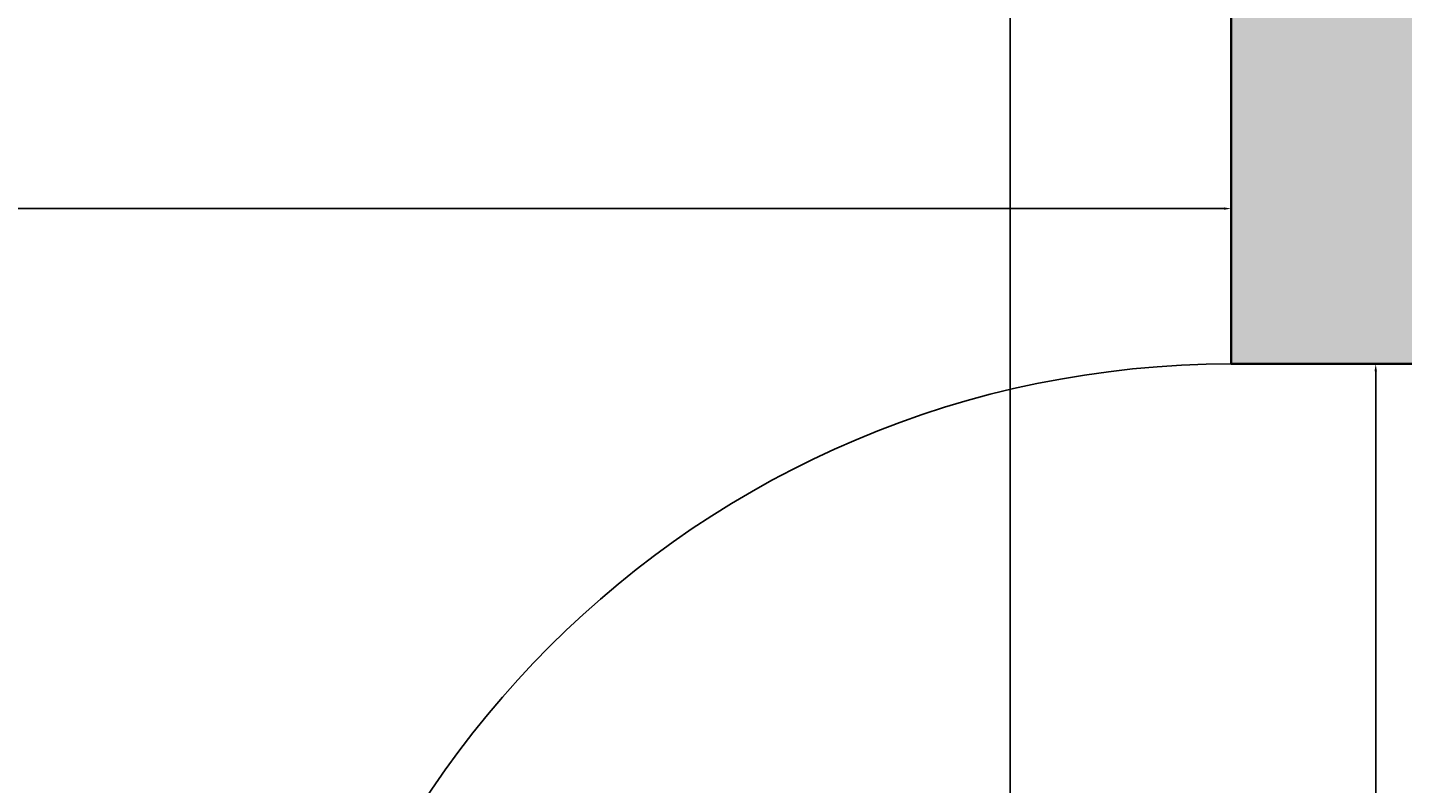
# Model space of a CAD drawing. Units: inches. Extents: x -5 to 482, y -460 to 66.
# Tile 20 of 31: x 120 to 154, y -124 to -105. Entities that reach past the tile are written whole.
import ezdxf

# ---------------------------------------------------------------- set-up
doc = ezdxf.new("R2010")
doc.units = ezdxf.units.IN
doc.header["$MEASUREMENT"] = 0
for name, color, linetype, lineweight in [('A-ANNO-DIMS', 2, 'Continuous', 18), ('A-DOOR', 3, 'Continuous', 25), ('A-WALL', 7, 'Continuous', 35), ('A-WALL-PATT', 152, 'Continuous', 13)]:
    doc.layers.add(name, color=color, linetype=linetype, lineweight=lineweight)
doc.styles.get("Standard").update_dxf_attribs({"font": 'arial.ttf'})
doc.dimstyles.get("Standard").update_dxf_attribs({"dimtxt": 0.18, "dimasz": 0.18, "dimexe": 0.18, "dimexo": 0.0625, "dimgap": 0.09, "dimtad": 0, "dimtih": 1, "dimtoh": 1, "dimdec": 0, "dimzin": 0, "dimdsep": 46, "dimlunit": 3, "dimtxsty": 'Standard', "dimcen": 0.09, "dimadec": 0, "dimazin": 0, "dimtfac": 1, "dimtdec": 0, "dimtofl": 0, "dimtmove": 0, "dimatfit": 3, "dimfxl": 1, "dimtolj": 1, "dimtzin": 0, "dimarcsym": 0})

# ---------------------------------------------------------------- blocks, each defined once
blk = doc.blocks.new('*D5')
at = {"layer": 'A-ANNO-DIMS', "color": 0, "lineweight": -2, "transparency": 16777216}
for p, q in [((41.877, -113.786), (41.877, -109.801)), ((42.057, -109.981), (93.026, -109.981)), ((149.697, -109.981), (98.727, -109.981)), ((149.877, -113.786), (149.877, -109.801))]:
    blk.add_line(p, q, dxfattribs=at)
at = {"layer": 'A-ANNO-DIMS', "color": 0, "transparency": 16777216}
for points in [[(42.057, -109.951), (42.057, -110.011), (41.877, -109.981)], [(149.697, -109.951), (149.697, -110.011), (149.877, -109.981)]]:
    blk.add_solid(points, dxfattribs=at)
at = {"layer": 'Defpoints', "color": 0, "transparency": 16777216}
for p in [(41.877, -109.981), (41.877, -113.849), (149.877, -113.849)]:
    blk.add_point(p, dxfattribs=at)
at = {"layer": 'A-ANNO-DIMS', "color": 0, "transparency": 16777216, "insert": (95.877, -109.981), "char_height": 6, "attachment_point": 5}
blk.add_mtext("\\A1;9'", dxfattribs=at)
blk = doc.blocks.new('DOOR-SWING-24IN')
for p, q in [((24, 1), (0, 1)), ((24, 0), (0, 0))]:
    blk.add_line(p, q)
blk.add_arc((24, 0), 24, 90, 180)
blk = doc.blocks.new('*D42')
at = {"layer": 'A-ANNO-DIMS', "color": 0, "lineweight": -2, "transparency": 16777216}
for p, q in [((149.939, -113.849), (153.657, -113.849)), ((153.477, -114.029), (153.477, -125.667)), ((153.477, -137.669), (153.477, -126.031)), ((149.939, -137.849), (153.657, -137.849))]:
    blk.add_line(p, q, dxfattribs=at)
at = {"layer": 'A-ANNO-DIMS', "color": 0, "transparency": 16777216}
for points in [[(153.447, -114.029), (153.507, -114.029), (153.477, -113.849)], [(153.447, -137.669), (153.507, -137.669), (153.477, -137.849)]]:
    blk.add_solid(points, dxfattribs=at)
at = {"layer": 'Defpoints', "color": 0, "transparency": 16777216}
for p in [(149.877, -113.849), (153.477, -113.849), (149.877, -137.849)]:
    blk.add_point(p, dxfattribs=at)
at = {"layer": 'A-ANNO-DIMS', "color": 0, "transparency": 16777216, "insert": (153.477, -125.849), "char_height": 0.18, "attachment_point": 5}
blk.add_mtext('\\A1;2\'-0" TYP.', dxfattribs=at)
blk = doc.blocks.new('*D73')
at = {"layer": 'A-ANNO-DIMS', "color": 0, "lineweight": -2, "transparency": 16777216}
for p, q in [((144.377, -295.799), (144.377, 50.931)), ((144.557, 50.751), (160.976, 50.751)), ((178.197, 50.751), (161.777, 50.751)), ((178.377, -295.799), (178.377, 50.931))]:
    blk.add_line(p, q, dxfattribs=at)
at = {"layer": 'A-ANNO-DIMS', "color": 0, "transparency": 16777216}
for points in [[(144.557, 50.781), (144.557, 50.721), (144.377, 50.751)], [(178.197, 50.781), (178.197, 50.721), (178.377, 50.751)]]:
    blk.add_solid(points, dxfattribs=at)
at = {"layer": 'Defpoints', "color": 0, "transparency": 16777216}
for p in [(178.377, 50.751), (144.377, -295.861), (178.377, -295.861)]:
    blk.add_point(p, dxfattribs=at)
at = {"layer": 'A-ANNO-DIMS', "color": 0, "transparency": 16777216, "insert": (161.377, 50.751), "char_height": 0.18, "attachment_point": 5}
blk.add_mtext('\\A1;2\'-10"', dxfattribs=at)

msp = doc.modelspace()

# ---------------------------------------------------------------- hatches: boundary and pattern name
at = {"layer": 'A-WALL-PATT'}
h = msp.add_hatch(color=256, dxfattribs=at)
h.dxf.hatch_style = 1
h.paths.add_polyline_path([(149.377, -412.849), (144.377, -412.849), (144.377, -283.849), (144.377, -279.349), (133.877, -279.349), (133.877, -283.849), (139.877, -283.849), (139.877, -412.849), (133.51, -412.849), (133.51, -413.916), (102.652, -413.916), (102.652, -421.02), (133.51, -421.02), (133.51, -421.849), (149.377, -421.849)])
h.paths.add_polyline_path([(226.054, -412.849), (218.877, -412.849), (218.877, -350.849), (262.877, -350.849), (262.877, -386.849), (267.377, -386.849), (267.377, -283.849), (270.377, -283.849), (270.377, -279.349), (244.877, -279.349), (244.877, -283.849), (262.877, -283.849), (262.877, -346.349), (218.877, -346.349), (218.877, -283.849), (220.877, -283.849), (220.877, -279.349), (214.377, -279.349), (214.377, -283.849), (214.377, -412.849), (209.377, -412.849), (209.377, -421.849), (226.054, -421.849)])
h.paths.add_polyline_path([(315.815, -412.849), (250.054, -412.849), (250.054, -421.849), (315.815, -421.849)])
h.paths.add_polyline_path([(430.377, -378.349), (421.377, -378.349), (421.377, -412.849), (375.815, -412.849), (375.815, -421.849), (430.377, -421.849)])
h.paths.add_polyline_path([(78.691, -413.916), (47.68, -413.916), (47.68, -412.849), (41.877, -412.849), (41.877, -283.849), (109.877, -283.849), (109.877, -279.349), (41.877, -279.349), (41.877, -241.849), (32.877, -241.849), (32.877, -421.849), (47.68, -421.849), (47.68, -421.02), (78.691, -421.02)])
h.paths.add_polyline_path([(41.877, -144.349), (154.377, -144.349), (154.377, -137.849), (149.877, -137.849), (149.877, -139.849), (41.877, -139.849), (41.877, -97.849), (32.877, -97.849), (32.877, -181.849), (41.877, -181.849)])
h.paths.add_polyline_path([(430.377, -241.849), (421.377, -241.849), (421.377, -279.349), (309.377, -279.349), (309.377, -170.349), (304.877, -170.349), (304.877, -279.349), (294.377, -279.349), (294.377, -283.849), (421.377, -283.849), (421.377, -318.349), (430.377, -318.349)])
h.paths.add_polyline_path([(430.377, -119.849), (421.377, -119.849), (421.377, -139.849), (419.377, -139.849), (419.377, -144.349), (421.377, -144.349), (421.377, -181.849), (430.377, -181.849)])
h.paths.add_polyline_path([(395.377, -139.849), (377.377, -139.849), (377.377, -75.849), (421.377, -75.849), (421.377, -95.849), (430.377, -95.849), (430.377, -45.599), (421.377, -45.599), (421.377, -71.349), (377.377, -71.349), (377.377, -22.849), (372.877, -22.849), (372.877, -139.849), (242.877, -139.849), (242.877, -137.849), (238.377, -137.849), (238.377, -144.349), (304.877, -144.349), (304.877, -146.349), (309.377, -146.349), (309.377, -144.349), (395.377, -144.349)])
h.paths.add_polyline_path([(65.877, 13.151), (32.877, 13.151), (32.877, -37.849), (41.877, -37.849), (41.877, 4.151), (65.877, 4.151)])
h.paths.add_polyline_path([(166.377, 13.151), (125.877, 13.151), (125.877, 4.151), (149.877, 4.151), (149.877, -113.849), (154.377, -113.849), (154.377, 4.151), (166.377, 4.151)])
h.paths.add_polyline_path([(277.877, 13.151), (226.377, 13.151), (226.377, 4.151), (238.377, 4.151), (238.377, -113.849), (242.877, -113.849), (242.877, 4.151), (277.877, 4.151)])
h.paths.add_polyline_path([(430.377, 13.151), (337.877, 13.151), (337.877, 4.151), (372.877, 4.151), (372.877, 1.151), (377.377, 1.151), (377.377, 4.151), (421.377, 4.151), (421.377, -21.599), (430.377, -21.599)])

# ---------------------------------------------------------------- linework, layer by layer
at = {"layer": 'A-WALL'}
for p, q in [((149.877, 4.151), (149.877, -113.849)), ((149.877, -113.849), (154.377, -113.849))]:
    msp.add_line(p, q, dxfattribs=at)

# ---------------------------------------------------------------- block references
at = {"layer": 'A-DOOR'}
msp.add_blockref('DOOR-SWING-24IN', (125.877, -137.849), dxfattribs=at)

# ---------------------------------------------------------------- dimensions: what is measured, and where the dimension line sits
at = {"layer": 'A-ANNO-DIMS'}
for base, p1, p2, override, picture, middle in [((178.377, 50.751), (144.377, -295.861), (178.377, -295.861), {"dimdec": 1, "dimlfac": 1, "dimrnd": 0, "dimzin": 1, "dimdsep": 46, "dimlunit": 4, "dimfrac": 2}, '*D73', (161.377, 50.751)), ((41.877, -109.981), (149.877, -113.849), (41.877, -113.849), {"dimtxt": 6, "dimclrd": 0, "dimclre": 0, "dimclrt": 0}, '*D5', (95.877, -109.981))]:
    dim = msp.add_linear_dim(base=base, p1=p1, p2=p2, dimstyle='Standard', override=override, dxfattribs=at)
    dim.commit()
    dim.dimension.update_dxf_attribs({"geometry": picture, "text_midpoint": middle})
dim = msp.add_linear_dim(base=(153.477, -113.849), p1=(149.877, -137.849), p2=(149.877, -113.849), angle=90, text='<> TYP.', dimstyle='Standard', override={"dimdec": 1, "dimlfac": 1, "dimrnd": 0, "dimzin": 1, "dimdsep": 46, "dimlunit": 4, "dimfrac": 2}, dxfattribs=at)
dim.commit()
dim.dimension.update_dxf_attribs({"geometry": '*D42', "text_midpoint": (153.477, -125.849)})

doc.saveas('drawing.dxf')
